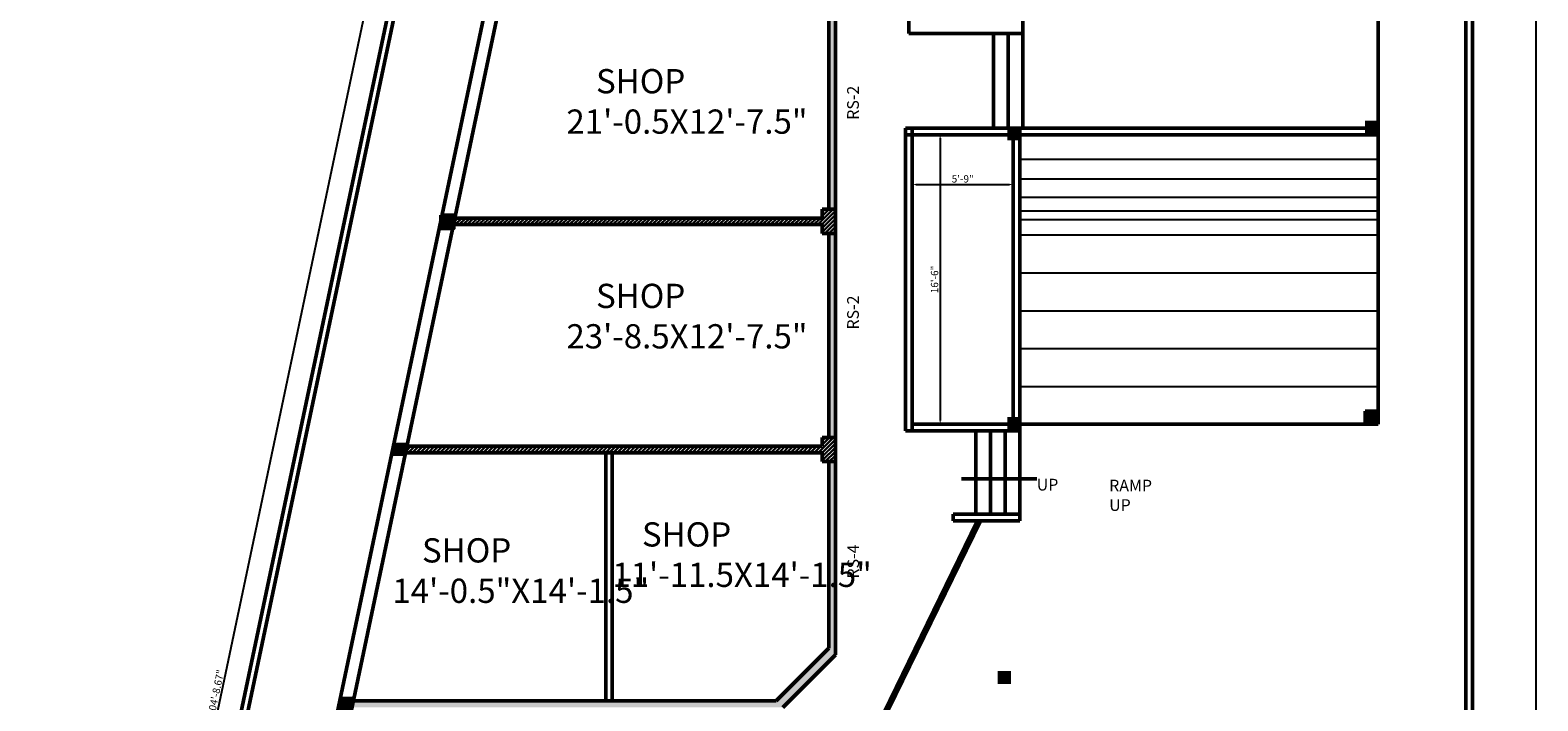
# Model space of a CAD drawing. Units: inches. Extents: x -2733 to 3435, y -338 to 1843.
# Tile 2 of 7: x -2733 to -1702, y 305 to 764. Entities that reach past the tile are written whole.
import ezdxf

# ---------------------------------------------------------------- set-up
doc = ezdxf.new("R2010")
doc.units = ezdxf.units.IN
doc.header["$PDMODE"] = 34
for name, color, linetype, lineweight in [('A-ANNO-DIMS', 2, 'Continuous', 18), ('A-ANNO-TEXT', 7, 'Continuous', 18), ('A-AREA-IDEN', 3, 'Continuous', 18), ('A-COLS', 1, 'Continuous', 35), ('A-FLOR-STRS', 4, 'Continuous', 25), ('A-WALL', 7, 'Continuous', 50), ('A-WALL-PATT', 8, 'Continuous', 13)]:
    doc.layers.add(name, color=color, linetype=linetype, lineweight=lineweight)
doc.styles.get("Standard").update_dxf_attribs({"font": 'arial.ttf'})
doc.styles.add('YQ_DIM', font='SUPEROS.SHX', dxfattribs={"width": 0.8, "bigfont": 'HZDX.SHX'})
doc.dimstyles.new('ISO-25', dxfattribs={"dimtxt": 5, "dimasz": 2.5, "dimexe": 1.25, "dimexo": 0.625, "dimtad": 1, "dimlunit": 3, "dimtxsty": 'Standard', "dimcen": 2.5, "dimadec": 0, "dimazin": 0, "dimtfac": 1, "dimtmove": 0, "dimatfit": 3, "dimfxl": 1, "dimarcsym": 0})

# ---------------------------------------------------------------- blocks, each defined once
blk = doc.blocks.new('*D5')
at = {"layer": 'A-ANNO-DIMS', "color": 0, "lineweight": -2, "transparency": 16777216}
for p, q in [((-2473, 922.1), (-2730.9, -302.7)), ((-2457.7, 921.4), (-2473.7, 924.8)), ((-2716.6, -308.3), (-2732.6, -304.9))]:
    blk.add_line(p, q, dxfattribs=at)
at = {"layer": 'A-ANNO-DIMS', "color": 0, "lineweight": 20, "transparency": 16777216}
for points in [[(-2473.4, 922.2), (-2472.6, 922), (-2472.5, 924.6)], [(-2731.3, -302.6), (-2730.5, -302.8), (-2731.4, -305.2)]]:
    blk.add_solid(points, dxfattribs=at)
at = {"layer": 'Defpoints', "color": 0, "lineweight": 20, "transparency": 16777216}
for p in [(-2457, 921.3), (-2731.4, -305.2), (-2715.9, -308.4)]:
    blk.add_point(p, dxfattribs=at)
at = {"layer": 'A-ANNO-DIMS', "color": 0, "transparency": 16777216, "insert": (-2605, 310.4), "char_height": 5, "attachment_point": 5, "rotation": 78.1108}
blk.add_mtext('104\'-8.67"', dxfattribs=at)
blk = doc.blocks.new('*D6')
at = {"layer": 'A-ANNO-DIMS', "color": 0, "lineweight": -2, "transparency": 16777216}
for p, q in [((-1745.9, 1560.1), (-1701.9, 1560.1)), ((-1703.2, 1557.6), (-1703.2, 266.6)), ((-1745.9, 264.1), (-1701.9, 264.1))]:
    blk.add_line(p, q, dxfattribs=at)
at = {"layer": 'A-ANNO-DIMS', "color": 0, "lineweight": 20, "transparency": 16777216}
for points in [[(-1703.6, 1557.6), (-1702.8, 1557.6), (-1703.2, 1560.1)], [(-1703.6, 266.6), (-1702.8, 266.6), (-1703.2, 264.1)]]:
    blk.add_solid(points, dxfattribs=at)
at = {"layer": 'Defpoints', "color": 0, "lineweight": 20, "transparency": 16777216}
for p in [(-1746.6, 1560.1), (-1746.6, 264.1), (-1703.2, 264.1)]:
    blk.add_point(p, dxfattribs=at)
at = {"layer": 'A-ANNO-DIMS', "color": 0, "transparency": 16777216, "insert": (-1706.4, 912.1), "char_height": 5, "attachment_point": 5, "rotation": 90}
blk.add_mtext("108'", dxfattribs=at)
blk = doc.blocks.new('*D10')
at = {"layer": 'A-ANNO-DIMS', "color": 0, "lineweight": -2, "transparency": 16777216}
for p, q in [((-2129.6, 658.7), (-2129.6, 659.3)), ((-2127.1, 658.1), (-2063.1, 658.1)), ((-2060.6, 658.7), (-2060.6, 659.3))]:
    blk.add_line(p, q, dxfattribs=at)
at = {"layer": 'A-ANNO-DIMS', "color": 0, "lineweight": 20, "transparency": 16777216}
for points in [[(-2127.1, 658.5), (-2127.1, 657.6), (-2129.6, 658.1)], [(-2063.1, 658.5), (-2063.1, 657.6), (-2060.6, 658.1)]]:
    blk.add_solid(points, dxfattribs=at)
at = {"layer": 'Defpoints', "color": 0, "lineweight": 20, "transparency": 16777216}
for p in [(-2129.6, 658.1), (-2060.6, 658.1), (-2060.6, 658.1)]:
    blk.add_point(p, dxfattribs=at)
at = {"layer": 'A-ANNO-DIMS', "color": 0, "transparency": 16777216, "insert": (-2095.1, 661.2), "char_height": 5, "attachment_point": 5}
blk.add_mtext('5\'-9"', dxfattribs=at)
blk = doc.blocks.new('*D11')
at = {"layer": 'A-ANNO-DIMS', "color": 0, "lineweight": -2, "transparency": 16777216}
for p, q in [((-2111, 692.1), (-2109.2, 692.1)), ((-2110.5, 689.6), (-2110.5, 496.6)), ((-2105.5, 494.1), (-2111.7, 494.1))]:
    blk.add_line(p, q, dxfattribs=at)
at = {"layer": 'A-ANNO-DIMS', "color": 0, "lineweight": 20, "transparency": 16777216}
for points in [[(-2110.9, 689.6), (-2110.1, 689.6), (-2110.5, 692.1)], [(-2110.9, 496.6), (-2110.1, 496.6), (-2110.5, 494.1)]]:
    blk.add_solid(points, dxfattribs=at)
at = {"layer": 'Defpoints', "color": 0, "lineweight": 20, "transparency": 16777216}
for p in [(-2111.6, 692.1), (-2110.5, 494.1), (-2104.8, 494.1)]:
    blk.add_point(p, dxfattribs=at)
at = {"layer": 'A-ANNO-DIMS', "color": 0, "transparency": 16777216, "insert": (-2113.7, 593.1), "char_height": 5, "attachment_point": 5, "rotation": 90}
blk.add_mtext('16\'-6"', dxfattribs=at)
blk = doc.blocks.new('*D22')
at = {"layer": 'A-ANNO-DIMS', "color": 0, "lineweight": -2, "transparency": 16777216}
blk.add_arc((-2457, 921.3), 20.3, 94.064, 251.0467, dxfattribs=at)
at = {"layer": 'A-ANNO-DIMS', "color": 0, "lineweight": 20, "transparency": 16777216}
for points in [[(-2458.5, 942), (-2458.5, 941.1), (-2456, 941.6)], [(-2463.5, 902.5), (-2463.7, 901.7), (-2461.2, 901.5)]]:
    blk.add_solid(points, dxfattribs=at)
at = {"layer": 'Defpoints', "color": 0, "lineweight": 20, "transparency": 16777216}
for p in [(-2423.6, 1560.1), (-2473.5, 933.2), (-2457, 921.3), (-2457, 921.3), (-2718.3, -319.8)]:
    blk.add_point(p, dxfattribs=at)
at = {"layer": 'A-ANNO-DIMS', "color": 0, "transparency": 16777216, "insert": (-2480.3, 924.3), "char_height": 5, "attachment_point": 5, "rotation": 82.5554}
blk.add_mtext('171°', dxfattribs=at)

msp = doc.modelspace()

# ---------------------------------------------------------------- hatches: boundary and pattern name
at = {"layer": 'A-COLS'}
h = msp.add_hatch(color=256, dxfattribs=at)
h.dxf.hatch_style = 1
h.paths.add_polyline_path([(-1811.069, 701.681), (-1820.069, 701.681), (-1820.069, 692.681), (-1811.069, 692.681)])
h = msp.add_hatch(color=256, dxfattribs=at)
h.dxf.hatch_style = 1
h.paths.add_polyline_path([(-2055.55, 697.181), (-2064.55, 697.181), (-2064.55, 688.181), (-2055.55, 688.181)])
h = msp.add_hatch(color=256, dxfattribs=at)
h.dxf.hatch_style = 1
h.paths.add_polyline_path([(-2442.925, 636.993), (-2450.993, 636.993), (-2451.925, 632.566), (-2451.925, 627.993), (-2443.773, 627.993), (-2442.925, 632.021)])
h = msp.add_hatch(color=256, dxfattribs=at)
h.dxf.hatch_style = 1
h.paths.add_polyline_path([(-2055.55, 499.181), (-2064.55, 499.181), (-2064.55, 490.181), (-2055.55, 490.181)])
h = msp.add_hatch(color=256, dxfattribs=at)
h.dxf.hatch_style = 1
h.paths.add_polyline_path([(-1811.069, 503.08), (-1820.069, 503.08), (-1820.069, 494.08), (-1811.069, 494.08)])
h = msp.add_hatch(color=256, dxfattribs=at)
h.dxf.hatch_style = 1
h.paths.add_polyline_path([(-2475.363, 481.44), (-2484.363, 481.44), (-2484.363, 472.44), (-2475.363, 472.44)])
h = msp.add_hatch(color=256, dxfattribs=at)
h.dxf.hatch_style = 1
h.paths.add_polyline_path([(-2062.151, 325.56), (-2071.151, 325.56), (-2071.151, 316.56), (-2062.151, 316.56)])
h = msp.add_hatch(color=256, dxfattribs=at)
h.dxf.hatch_style = 1
h.paths.add_polyline_path([(-2512.158, 307.862), (-2521.158, 307.862), (-2521.158, 298.862), (-2512.158, 298.862)])
at = {"layer": 'A-WALL-PATT'}
h = msp.add_hatch(color=256, dxfattribs=at)
h.dxf.hatch_style = 1
h.paths.add_polyline_path([(-2182.126, 776.08), (-2186.626, 776.08), (-2186.626, 641.08), (-2182.126, 641.08)])
h.paths.add_polyline_path([(-2182.126, 932.085), (-2186.626, 932.085), (-2186.626, 792.58), (-2182.126, 792.58)])
h.paths.add_polyline_path([(-2182.126, 624.58), (-2186.626, 624.58), (-2186.626, 485.101), (-2182.126, 485.101)])
h.paths.add_polyline_path([(-2182.126, 468.606), (-2186.626, 468.606), (-2186.626, 341.08), (-2222.626, 305.08), (-2511.726, 305.08), (-2512.673, 300.58), (-2218.126, 300.58), (-2182.126, 336.58)])
h.paths.add_polyline_path([(-2182.126, 1088.154), (-2186.626, 1088.154), (-2186.626, 948.58), (-2182.126, 948.582)])
h.paths.add_polyline_path([(-2182.126, 1243.861), (-2186.626, 1243.861), (-2186.626, 1104.649), (-2182.126, 1104.649)])
h.paths.add_polyline_path([(-2182.126, 1340.024), (-2186.626, 1340.024), (-2186.626, 1260.356), (-2182.126, 1260.356)])
h.paths.add_polyline_path([(-2182.126, 1508.58), (-2186.626, 1508.58), (-2186.626, 1356.519), (-2182.126, 1356.519)])
h = msp.add_hatch(dxfattribs=at)
h.set_pattern_fill('ANSI32', color=256, scale=0.2)
h.set_pattern_definition([(45, (-2862.9097, 0), (-1.3470384, 1.3470384), []), (45, (-2862.0116, 0), (-1.3470384, 1.3470384), [])])
h.paths.add_polyline_path([(-2182.126, 641.08), (-2186.626, 641.08), (-2186.626, 641.075), (-2191.126, 641.075), (-2191.126, 635.08), (-2442.281, 635.08), (-2443.228, 630.58), (-2191.126, 630.58), (-2191.126, 624.58), (-2186.626, 624.58), (-2182.126, 624.58)])
h.paths.add_polyline_path([(-2182.126, 1104.649), (-2191.126, 1104.649), (-2191.126, 1098.58), (-2374.156, 1098.58), (-2374.392, 1094.08), (-2191.126, 1094.08), (-2191.126, 1088.154), (-2182.126, 1088.154)])
h.paths.add_polyline_path([(-2182.126, 948.58), (-2186.626, 948.58), (-2191.126, 948.58), (-2191.126, 942.58), (-2382.332, 942.58), (-2382.556, 938.295), (-2191.126, 938.09), (-2191.126, 932.085), (-2186.626, 932.085), (-2182.126, 932.085)])
h.paths.add_polyline_path([(-2182.126, 485.101), (-2191.126, 485.101), (-2191.126, 479.08), (-2475.11, 479.08), (-2476.057, 474.58), (-2191.126, 474.58), (-2191.126, 468.606), (-2182.126, 468.606)])
h.paths.add_polyline_path([(-2182.126, 792.575), (-2192.673, 792.575), (-2192.673, 786.58), (-2410.4, 786.58), (-2411.347, 782.08), (-2192.673, 782.08), (-2192.673, 776.08), (-2186.626, 776.08), (-2182.126, 776.08)])

# ---------------------------------------------------------------- linework, layer by layer
at = {"layer": 'A-FLOR-STRS'}
for p, q in [((-2056.126, 675.295), (-1811.069, 675.295)), ((-2056.126, 661.784), (-1811.069, 661.784)), ((-2056.126, 649.407), (-1811.069, 649.407)), ((-2056.126, 640.05), (-1811.069, 640.05)), ((-1811.069, 633.78), (-2056.126, 633.78)), ((-2056.126, 623.519), (-1811.069, 623.519)), ((-2056.126, 597.631), (-1811.069, 597.631)), ((-2056.126, 571.744), (-1811.069, 571.744)), ((-2056.126, 545.856), (-1811.069, 545.856)), ((-2056.126, 519.968), (-1811.069, 519.968))]:
    msp.add_line(p, q, dxfattribs=at)
at = {"layer": 'A-WALL'}
for p, q in [((-1746.569, 1560.127), (-1746.569, 264.127)), ((-1751.069, 1555.627), (-1751.069, 266.673)), ((-1811.069, 1517.58), (-1811.069, 503.08)), ((-1811.069, 1517.58), (-1811.069, 513.58)), ((-2182.126, 1508.58), (-2182.126, 336.58)), ((-2132.006, 1156.269), (-2132.006, 761.269)), ((-2054.006, 1156.269), (-2054.006, 761.269)), ((-2718.342, -319.774), (-2457.047, 921.314)), ((-2711.812, -310.6), (-2452.644, 920.386)), ((-2528.543, 268.651), (-2392.898, 912.931)), ((-2518.444, 273.153), (-2383.91, 912.46)), ((-2186.626, 776.08), (-2186.626, 641.075)), ((-2132.006, 761.269), (-2054.006, 761.269)), ((-2074.006, 761.269), (-2074.006, 696.58)), ((-2064.006, 696.58), (-2064.006, 761.269)), ((-2054.006, 761.269), (-2054.006, 696.58)), ((-1746.569, 264.127), (-1746.569, 729.127)), ((-2134.126, 696.58), (-1811.069, 696.58)), ((-2134.126, 696.58), (-2134.126, 692.08)), ((-2134.126, 696.58), (-2134.126, 489.58)), ((-2134.126, 692.08), (-1811.069, 692.08)), ((-2129.626, 696.58), (-2129.626, 489.58)), ((-2060.626, 696.58), (-2060.626, 489.58)), ((-2056.126, 696.58), (-2056.126, 489.58)), ((-2191.126, 635.075), (-2191.126, 641.075)), ((-2191.126, 641.075), (-2186.626, 641.075)), ((-2186.626, 641.08), (-2182.126, 641.08)), ((-1811.069, 640.05), (-1811.069, 633.78)), ((-2443.146, 630.58), (-2191.126, 630.58)), ((-2442.199, 635.08), (-2191.126, 635.08)), ((-2191.126, 624.58), (-2191.126, 630.585)), ((-2186.626, 624.58), (-2191.126, 624.58)), ((-2186.626, 624.58), (-2186.626, 485.101)), ((-2186.626, 624.58), (-2182.126, 624.58)), ((-1811.069, 503.08), (-1820.069, 503.08)), ((-1820.069, 503.08), (-1820.069, 494.08)), ((-1811.069, 494.08), (-1811.069, 503.08)), ((-2191.126, 479.08), (-2191.126, 485.101)), ((-2191.126, 485.101), (-2182.126, 485.101)), ((-2129.626, 489.58), (-2134.126, 489.58)), ((-2129.626, 494.08), (-2056.126, 494.08)), ((-2129.626, 489.58), (-2056.126, 489.58)), ((-2086.126, 489.58), (-2086.126, 432.58)), ((-2076.126, 489.58), (-2076.126, 432.58)), ((-2066.126, 489.58), (-2066.126, 432.58)), ((-2056.126, 494.08), (-1811.069, 494.08)), ((-2056.126, 489.58), (-2056.126, 432.58)), ((-1820.069, 494.08), (-1811.069, 494.08)), ((-2475.99, 474.58), (-2191.126, 474.58)), ((-2475.042, 479.08), (-2191.126, 479.08)), ((-2339.126, 474.58), (-2339.126, 305.08)), ((-2334.626, 474.58), (-2334.626, 305.08)), ((-2191.126, 468.606), (-2191.126, 474.611)), ((-2182.126, 468.606), (-2191.126, 468.606)), ((-2186.626, 468.606), (-2186.626, 341.08)), ((-2044.507, 456.848), (-2095.946, 456.848)), ((-2160.689, 273.202), (-2085.203, 428.08)), ((-2160.689, 268.702), (-2082.673, 428.08)), ((-2056.126, 432.58), (-2101.586, 432.58)), ((-2101.586, 432.58), (-2101.586, 428.08)), ((-2101.586, 428.08), (-2056.126, 428.08)), ((-2056.126, 428.08), (-2056.126, 432.58)), ((-2222.626, 305.08), (-2186.626, 341.08)), ((-2218.126, 300.58), (-2182.126, 336.58)), ((-2511.726, 305.08), (-2222.626, 305.08))]:
    msp.add_line(p, q, dxfattribs=at)
msp.add_lwpolyline([(-2451.925, 636.993), (-2442.925, 636.993), (-2442.925, 627.993), (-2451.925, 627.993)], close=True, dxfattribs=at)

# ---------------------------------------------------------------- texts
at = {"layer": 'A-ANNO-TEXT', "char_height": 8, "attachment_point": 1, "rotation": 90, "style": 'YQ_DIM'}
for s, insert in [('{\\fSwis721 BlkCn BT|b0|i0|c0|p34;RS-2}', (-2174.09, 702.242)), ('{\\fSwis721 BlkCn BT|b0|i0|c0|p34;RS-2}', (-2174.09, 558.851)), ('{\\fSwis721 BlkCn BT|b0|i0|c0|p34;RS-4}', (-2173.963, 388.652))]:
    msp.add_mtext_dynamic_manual_height_columns(s, width=14.9584, gutter_width=12.5, heights=[0], dxfattribs=dict(at, insert=insert))
at = {"layer": 'A-ANNO-TEXT', "char_height": 8, "attachment_point": 1, "style": 'YQ_DIM'}
for s, width, insert in [('{\\fSitka Banner Semibold|b1|i0|c0|p2;UP}', 3.68944, (-2044.507, 456.848)), ('{\\fSTZhongsong|b1|i0|c0|p2;RAMP UP}', 45.72976, (-1994.986, 456.218))]:
    msp.add_mtext_dynamic_manual_height_columns(s, width=width, gutter_width=12.5, heights=[0], dxfattribs=dict(at, insert=insert))
at = {"layer": 'A-AREA-IDEN', "char_height": 16.56819, "attachment_point": 1, "style": 'YQ_DIM'}
for s, insert in [('{\\f@SimSun|b1|i0|c0|p2; \\f@Arial Unicode MS|b1|i0|c0|p34;   SHOP\\P21\'-0.5X12\'-7.5\\f@SimSun|b1|i0|c0|p2;"}', (-2366.027, 736.918)), ('{\\f@SimSun|b1|i0|c0|p2; \\f@Arial Unicode MS|b1|i0|c0|p34;   SHOP\\P23\'-8.5X12\'-7.5\\f@SimSun|b1|i0|c0|p2;"}', (-2366.027, 590.151)), ('{\\f@SimSun|b1|i0|c0|p2; \\f@Arial Unicode MS|b1|i0|c0|p34;   SHOP\\P11\'-11.5X14\'-1.5\\f@SimSun|b1|i0|c0|p2;"}', (-2334.626, 427.124)), ('{\\f@SimSun|b1|i0|c0|p2; \\f@Arial Unicode MS|b1|i0|c0|p34;   SHOP\\P14\'-0.5"X14\'-1.5\\f@SimSun|b1|i0|c0|p2;"}', (-2485.001, 416.211))]:
    msp.add_mtext_dynamic_manual_height_columns(s, width=128.94034, gutter_width=26.518, heights=[0], dxfattribs=dict(at, insert=insert))

# ---------------------------------------------------------------- dimensions: what is measured, and where the dimension line sits
at = {"layer": 'A-ANNO-DIMS'}
dim = msp.add_angular_dim_2l(base=(-2473.47, 933.229), line1=((-2718.342, -319.774), (-2457.047, 921.314)), line2=((-2457.047, 921.314), (-2423.568, 1560.127)), dimstyle='ISO-25', override={"dimclrd": 0, "dimclre": 0, "dimclrt": 0}, dxfattribs=at)
dim.commit()
dim.dimension.update_dxf_attribs({"geometry": '*D22', "text_midpoint": (-2480.275, 924.349)})
for base, p1, p2, picture, middle in [((-1703.179, 264.127), (-1746.569, 1560.127), (-1746.569, 264.127), '*D6', (-1706.357, 912.127)), ((-2110.478, 494.08), (-2111.604, 692.08), (-2104.849, 494.08), '*D11', (-2113.656, 593.08))]:
    dim = msp.add_linear_dim(base=base, p1=p1, p2=p2, angle=90, dimstyle='ISO-25', override={"dimclrd": 0, "dimclre": 0, "dimclrt": 0}, dxfattribs=at)
    dim.commit()
    dim.dimension.update_dxf_attribs({"geometry": picture, "text_midpoint": middle})
dim = msp.add_aligned_dim(p1=(-2457.047, 921.314), p2=(-2715.948, -308.402), distance=-15.77, dimstyle='ISO-25', override={"dimclrd": 0, "dimclre": 0, "dimclrt": 0}, dxfattribs=at)
dim.commit()
dim.dimension.update_dxf_attribs({"geometry": '*D5', "text_midpoint": (-2605.039, 310.359)})
dim = msp.add_linear_dim(base=(-2060.626, 658.063), p1=(-2129.626, 658.063), p2=(-2060.626, 658.063), dimstyle='ISO-25', override={"dimclrd": 0, "dimclre": 0, "dimclrt": 0}, dxfattribs=at)
dim.commit()
dim.dimension.update_dxf_attribs({"geometry": '*D10', "text_midpoint": (-2095.126, 661.241)})

doc.saveas('drawing.dxf')
